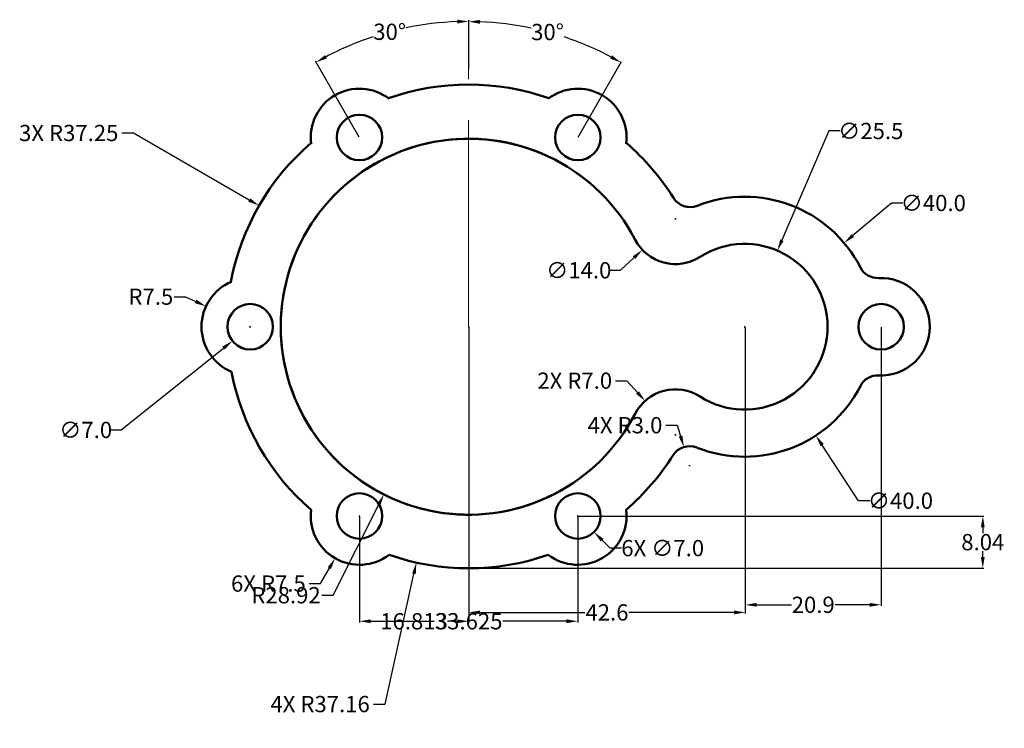
# Model space of a CAD drawing. Units: millimetres. Extents: x -471 to -319, y 2 to 111.
import ezdxf

# ---------------------------------------------------------------- set-up
doc = ezdxf.new("R2010")
doc.units = ezdxf.units.MM
doc.header["$MEASUREMENT"] = 0
doc.linetypes.add('CENTER', pattern=[50.8, 31.75, -6.35, 6.35, -6.35])
for name, color, linetype, lineweight in [('M-CNTR', 4, 'CENTER', 18), ('M-DIMS', 2, 'Continuous', 25), ('M-OUTL', 7, 'Continuous', 50)]:
    doc.layers.add(name, color=color, linetype=linetype, lineweight=lineweight)
doc.styles.get("Standard").update_dxf_attribs({"font": 'arial.ttf'})
doc.dimstyles.get("Standard").update_dxf_attribs({"dimtxt": 2.5, "dimasz": 1.75, "dimexe": 0.18, "dimexo": 0.0625, "dimgap": 0.09, "dimtad": 0, "dimtih": 1, "dimtoh": 1, "dimdec": 1, "dimzin": 0, "dimdsep": 46, "dimtxsty": 'Standard', "dimcen": 0.09, "dimadec": 0, "dimazin": 0, "dimtfac": 1, "dimtdec": 1, "dimtofl": 0, "dimtmove": 0, "dimatfit": 3, "dimfxl": 1, "dimtolj": 1, "dimtzin": 0, "dimarcsym": 0})

# ---------------------------------------------------------------- blocks, each defined once
blk = doc.blocks.new('*D1')
at = {"layer": 'Defpoints', "color": 0, "transparency": 16777216}
for p in [(-442.39, 67.1), (-435.58, 63.95)]:
    blk.add_point(p, dxfattribs=at)
at = {"layer": 'M-DIMS', "color": 0, "lineweight": -2, "transparency": 16777216}
for p, q in [((-447.31, 68.57), (-445.56, 68.57)), ((-445.56, 68.57), (-443.97, 67.83)), ((-435.67, 63.95), (-435.49, 63.95)), ((-435.58, 63.86), (-435.58, 64.04))]:
    blk.add_line(p, q, dxfattribs=at)
at = {"layer": 'M-DIMS', "color": 0, "transparency": 16777216}
blk.add_solid([(-443.85, 68.1), (-444.1, 67.57), (-442.39, 67.1)], dxfattribs=at)
at = {"layer": 'M-DIMS', "color": 0, "transparency": 16777216, "insert": (-450.88, 68.57), "char_height": 2.5, "attachment_point": 5}
blk.add_mtext('\\A1;R7.5', dxfattribs=at)
blk = doc.blocks.new('*D2')
at = {"layer": 'Defpoints', "color": 0, "transparency": 16777216}
for p in [(-432.85, 66.13), (-438.31, 61.76)]:
    blk.add_point(p, dxfattribs=at)
at = {"layer": 'M-DIMS', "color": 0, "lineweight": -2, "transparency": 16777216}
for p, q in [((-435.67, 63.95), (-435.49, 63.95)), ((-435.58, 63.86), (-435.58, 64.04)), ((-455.44, 48.07), (-439.68, 60.67)), ((-457.19, 48.07), (-455.44, 48.07))]:
    blk.add_line(p, q, dxfattribs=at)
at = {"layer": 'M-DIMS', "color": 0, "transparency": 16777216}
blk.add_solid([(-439.86, 60.9), (-439.5, 60.44), (-438.31, 61.76)], dxfattribs=at)
at = {"layer": 'M-DIMS', "color": 0, "transparency": 16777216, "insert": (-460.91, 48.07), "char_height": 2.5, "attachment_point": 5}
blk.add_mtext('\\A1;∅7.0', dxfattribs=at)
blk = doc.blocks.new('*D3')
at = {"layer": 'Defpoints', "color": 0, "transparency": 16777216}
for p in [(-365.02, 85.37), (-375.21, 75.78)]:
    blk.add_point(p, dxfattribs=at)
at = {"layer": 'M-DIMS', "color": 0, "lineweight": -2, "transparency": 16777216}
for p, q in [((-370.2, 80.57), (-370.02, 80.57)), ((-370.11, 80.48), (-370.11, 80.66)), ((-378.56, 72.63), (-376.49, 74.58)), ((-380.31, 72.63), (-378.56, 72.63))]:
    blk.add_line(p, q, dxfattribs=at)
at = {"layer": 'M-DIMS', "color": 0, "transparency": 16777216}
blk.add_solid([(-376.69, 74.79), (-376.29, 74.37), (-375.21, 75.78)], dxfattribs=at)
at = {"layer": 'M-DIMS', "color": 0, "transparency": 16777216, "insert": (-385, 72.63), "char_height": 2.5, "attachment_point": 5}
blk.add_mtext('\\A1;∅14.0', dxfattribs=at)
blk = doc.blocks.new('*D4')
at = {"layer": 'Defpoints', "color": 0, "transparency": 16777216}
for p in [(-354.42, 75.66), (-364.49, 52.24)]:
    blk.add_point(p, dxfattribs=at)
at = {"layer": 'M-DIMS', "color": 0, "lineweight": -2, "transparency": 16777216}
for p, q in [((-346.5, 94.06), (-353.72, 77.27)), ((-344.75, 94.06), (-346.5, 94.06)), ((-359.54, 63.95), (-359.36, 63.95)), ((-359.45, 63.86), (-359.45, 64.04))]:
    blk.add_line(p, q, dxfattribs=at)
at = {"layer": 'M-DIMS', "color": 0, "transparency": 16777216}
blk.add_solid([(-353.99, 77.38), (-353.46, 77.15), (-354.42, 75.66)], dxfattribs=at)
at = {"layer": 'M-DIMS', "color": 0, "transparency": 16777216, "insert": (-340.05, 94.06), "char_height": 2.5, "attachment_point": 5}
blk.add_mtext('\\A1;∅25.5', dxfattribs=at)
blk = doc.blocks.new('*D5')
at = {"layer": 'Defpoints', "color": 0, "transparency": 16777216}
for p in [(-344.16, 76.83), (-374.75, 51.06)]:
    blk.add_point(p, dxfattribs=at)
at = {"layer": 'M-DIMS', "color": 0, "lineweight": -2, "transparency": 16777216}
for p, q in [((-336.86, 82.98), (-342.82, 77.96)), ((-335.11, 82.98), (-336.86, 82.98)), ((-359.54, 63.95), (-359.36, 63.95)), ((-359.45, 63.86), (-359.45, 64.04))]:
    blk.add_line(p, q, dxfattribs=at)
at = {"layer": 'M-DIMS', "color": 0, "transparency": 16777216}
blk.add_solid([(-343.01, 78.18), (-342.63, 77.74), (-344.16, 76.83)], dxfattribs=at)
at = {"layer": 'M-DIMS', "color": 0, "transparency": 16777216, "insert": (-330.42, 82.98), "char_height": 2.5, "attachment_point": 5}
blk.add_mtext('\\A1;∅40.0', dxfattribs=at)
blk = doc.blocks.new('*D6')
at = {"layer": 'Defpoints', "color": 0, "transparency": 16777216}
for p in [(-401.95, 63.95), (-359.36, 63.95), (-359.36, 20)]:
    blk.add_point(p, dxfattribs=at)
at = {"layer": 'M-DIMS', "color": 0, "lineweight": -2, "transparency": 16777216}
for p, q in [((-401.95, 63.89), (-401.95, 19.82)), ((-359.36, 63.89), (-359.36, 19.82)), ((-400.2, 20), (-384.05, 20)), ((-361.11, 20), (-377.27, 20))]:
    blk.add_line(p, q, dxfattribs=at)
at = {"layer": 'M-DIMS', "color": 0, "transparency": 16777216}
for points in [[(-400.2, 20.29), (-400.2, 19.71), (-401.95, 20)], [(-361.11, 20.29), (-361.11, 19.71), (-359.36, 20)]]:
    blk.add_solid(points, dxfattribs=at)
at = {"layer": 'M-DIMS', "color": 0, "transparency": 16777216, "insert": (-380.66, 20), "char_height": 2.5, "attachment_point": 5}
blk.add_mtext('\\A1;42.6', dxfattribs=at)
blk = doc.blocks.new('*D7')
at = {"layer": 'Defpoints', "color": 0, "transparency": 16777216}
for p in [(-359.36, 63.95), (-338.45, 63.95), (-338.45, 21.17)]:
    blk.add_point(p, dxfattribs=at)
at = {"layer": 'M-DIMS', "color": 0, "lineweight": -2, "transparency": 16777216}
for p, q in [((-359.36, 63.89), (-359.36, 20.99)), ((-338.45, 63.89), (-338.45, 20.99)), ((-357.61, 21.17), (-352.27, 21.17)), ((-340.2, 21.17), (-345.55, 21.17))]:
    blk.add_line(p, q, dxfattribs=at)
at = {"layer": 'M-DIMS', "color": 0, "transparency": 16777216}
for points in [[(-357.61, 21.46), (-357.61, 20.88), (-359.36, 21.17)], [(-340.2, 21.46), (-340.2, 20.88), (-338.45, 21.17)]]:
    blk.add_solid(points, dxfattribs=at)
at = {"layer": 'M-DIMS', "color": 0, "transparency": 16777216, "insert": (-348.91, 21.17), "char_height": 2.5, "attachment_point": 5}
blk.add_mtext('\\A1;20.9', dxfattribs=at)
blk = doc.blocks.new('*D8')
at = {"layer": 'Defpoints', "color": 0, "transparency": 16777216}
for p in [(-410.11, 110.21), (-401.95, 103.42), (-418.77, 93.07), (-401.95, 63.95), (-401.95, 63.95)]:
    blk.add_point(p, dxfattribs=at)
at = {"layer": 'M-DIMS', "color": 0, "lineweight": -2, "transparency": 16777216}
for p, q in [((-401.95, 103.49), (-401.95, 111.1)), ((-418.8, 93.12), (-425.53, 104.78))]:
    blk.add_line(p, q, dxfattribs=at)
for start, end in [(92.1348, 101.8127), (108.2356, 117.8652)]:
    blk.add_arc((-401.95, 63.95), 46.97, start, end, dxfattribs=at)
at = {"layer": 'M-DIMS', "color": 0, "transparency": 16777216}
for points in [[(-403.71, 111.18), (-403.7, 110.59), (-401.95, 110.92)], [(-423.77, 105.22), (-424.05, 105.73), (-425.44, 104.63)]]:
    blk.add_solid(points, dxfattribs=at)
at = {"layer": 'M-DIMS', "color": 0, "transparency": 16777216, "insert": (-414.11, 109.32), "char_height": 2.5, "attachment_point": 5}
blk.add_mtext('\\A1;30°', dxfattribs=at)
blk = doc.blocks.new('*D9')
at = {"layer": 'Defpoints', "color": 0, "transparency": 16777216}
for p in [(-385.9, 108.05), (-401.95, 103.42), (-385.14, 93.07), (-401.95, 63.95), (-401.95, 63.95)]:
    blk.add_point(p, dxfattribs=at)
at = {"layer": 'M-DIMS', "color": 0, "lineweight": -2, "transparency": 16777216}
for p, q in [((-401.95, 103.49), (-401.95, 111.06)), ((-385.11, 93.12), (-378.4, 104.75))]:
    blk.add_line(p, q, dxfattribs=at)
for start, end in [(78.19, 87.8633), (62.1367, 71.7616)]:
    blk.add_arc((-401.95, 63.95), 46.93, start, end, dxfattribs=at)
at = {"layer": 'M-DIMS', "color": 0, "transparency": 16777216}
for points in [[(-400.21, 110.55), (-400.2, 111.14), (-401.95, 110.88)], [(-379.88, 105.69), (-380.16, 105.18), (-378.49, 104.59)]]:
    blk.add_solid(points, dxfattribs=at)
at = {"layer": 'M-DIMS', "color": 0, "transparency": 16777216, "insert": (-389.81, 109.28), "char_height": 2.5, "attachment_point": 5}
blk.add_mtext('\\A1;30°', dxfattribs=at)
blk = doc.blocks.new('MOUNTING-TAB-D7-R7_5')
blk.add_circle((0, 0), 3.5)
blk.add_arc((0, 0), 7.5, 112.6198, 247.3802)
blk = doc.blocks.new('*D11')
at = {"layer": 'Defpoints', "color": 0, "transparency": 16777216}
for p in [(-418.77, 34.83), (-385.14, 34.83), (-385.14, 18.64)]:
    blk.add_point(p, dxfattribs=at)
at = {"layer": 'M-DIMS', "color": 0, "lineweight": -2, "transparency": 16777216}
for p, q in [((-418.77, 34.77), (-418.77, 18.46)), ((-385.14, 34.77), (-385.14, 18.46)), ((-417.02, 18.64), (-407.24, 18.64)), ((-386.89, 18.64), (-396.67, 18.64))]:
    blk.add_line(p, q, dxfattribs=at)
at = {"layer": 'M-DIMS', "color": 0, "transparency": 16777216}
for points in [[(-417.02, 18.93), (-417.02, 18.35), (-418.77, 18.64)], [(-386.89, 18.93), (-386.89, 18.35), (-385.14, 18.64)]]:
    blk.add_solid(points, dxfattribs=at)
at = {"layer": 'M-DIMS', "color": 0, "transparency": 16777216, "insert": (-401.95, 18.64), "char_height": 2.5, "attachment_point": 5}
blk.add_mtext('\\A1;33.625', dxfattribs=at)
blk = doc.blocks.new('*D12')
at = {"layer": 'Defpoints', "color": 0, "transparency": 16777216}
for p in [(-418.77, 34.83), (-401.95, 26.79), (-401.95, 18.64)]:
    blk.add_point(p, dxfattribs=at)
at = {"layer": 'M-DIMS', "color": 0, "lineweight": -2, "transparency": 16777216}
for p, q in [((-418.77, 34.77), (-418.77, 18.46)), ((-401.95, 26.73), (-401.95, 18.46)), ((-417.02, 18.64), (-415.52, 18.64)), ((-403.7, 18.64), (-405.2, 18.64))]:
    blk.add_line(p, q, dxfattribs=at)
at = {"layer": 'M-DIMS', "color": 0, "transparency": 16777216}
for points in [[(-417.02, 18.93), (-417.02, 18.35), (-418.77, 18.64)], [(-403.7, 18.93), (-403.7, 18.35), (-401.95, 18.64)]]:
    blk.add_solid(points, dxfattribs=at)
at = {"layer": 'M-DIMS', "color": 0, "transparency": 16777216, "insert": (-410.36, 18.64), "char_height": 2.5, "attachment_point": 5}
blk.add_mtext('\\A1;16.813', dxfattribs=at)
blk = doc.blocks.new('*D13')
at = {"layer": 'Defpoints', "color": 0, "transparency": 16777216}
for p in [(-385.14, 34.83), (-401.95, 26.79), (-322.8, 26.79)]:
    blk.add_point(p, dxfattribs=at)
at = {"layer": 'M-DIMS', "color": 0, "lineweight": -2, "transparency": 16777216}
for p, q in [((-385.08, 34.83), (-322.62, 34.83)), ((-322.8, 33.08), (-322.8, 32.17)), ((-322.8, 28.54), (-322.8, 29.44)), ((-401.89, 26.79), (-322.62, 26.79))]:
    blk.add_line(p, q, dxfattribs=at)
at = {"layer": 'M-DIMS', "color": 0, "transparency": 16777216}
for points in [[(-323.1, 33.08), (-322.51, 33.08), (-322.8, 34.83)], [(-323.1, 28.54), (-322.51, 28.54), (-322.8, 26.79)]]:
    blk.add_solid(points, dxfattribs=at)
at = {"layer": 'M-DIMS', "color": 0, "transparency": 16777216, "insert": (-322.8, 30.81), "char_height": 2.5, "attachment_point": 5}
blk.add_mtext('\\A1;8.04', dxfattribs=at)
blk = doc.blocks.new('*D14')
at = {"layer": 'Defpoints', "color": 0, "transparency": 16777216}
for p in [(-387.62, 37.3), (-382.66, 32.36)]:
    blk.add_point(p, dxfattribs=at)
at = {"layer": 'M-DIMS', "color": 0, "lineweight": -2, "transparency": 16777216}
for p, q in [((-385.14, 34.74), (-385.14, 34.92)), ((-385.23, 34.83), (-385.05, 34.83)), ((-380.18, 29.89), (-381.42, 31.13)), ((-378.43, 29.89), (-380.18, 29.89))]:
    blk.add_line(p, q, dxfattribs=at)
at = {"layer": 'M-DIMS', "color": 0, "transparency": 16777216}
blk.add_solid([(-381.21, 31.33), (-381.63, 30.92), (-382.66, 32.36)], dxfattribs=at)
at = {"layer": 'M-DIMS', "color": 0, "transparency": 16777216, "insert": (-372.08, 29.89), "char_height": 2.5, "attachment_point": 5}
blk.add_mtext('\\A1;6X ∅7.0', dxfattribs=at)
blk = doc.blocks.new('*D15')
at = {"layer": 'Defpoints', "color": 0, "transparency": 16777216}
for p in [(-418.77, 34.83), (-422.52, 28.33)]:
    blk.add_point(p, dxfattribs=at)
at = {"layer": 'M-DIMS', "color": 0, "lineweight": -2, "transparency": 16777216}
for p, q in [((-418.77, 34.74), (-418.77, 34.92)), ((-418.86, 34.83), (-418.68, 34.83)), ((-424.77, 24.44), (-423.39, 26.82)), ((-426.52, 24.44), (-424.77, 24.44))]:
    blk.add_line(p, q, dxfattribs=at)
at = {"layer": 'M-DIMS', "color": 0, "transparency": 16777216}
blk.add_solid([(-423.65, 26.96), (-423.14, 26.67), (-422.52, 28.33)], dxfattribs=at)
at = {"layer": 'M-DIMS', "color": 0, "transparency": 16777216, "insert": (-432.78, 24.44), "char_height": 2.5, "attachment_point": 5}
blk.add_mtext('\\A1;6X R7.5', dxfattribs=at)
blk = doc.blocks.new('*D16')
at = {"layer": 'Defpoints', "color": 0, "transparency": 16777216}
for p in [(-434.21, 82.57), (-401.95, 63.95)]:
    blk.add_point(p, dxfattribs=at)
at = {"layer": 'M-DIMS', "color": 0, "lineweight": -2, "transparency": 16777216}
for p, q in [((-455.32, 93.75), (-453.57, 93.75)), ((-453.57, 93.75), (-435.73, 83.45)), ((-402.04, 63.95), (-401.86, 63.95)), ((-401.95, 63.86), (-401.95, 64.04))]:
    blk.add_line(p, q, dxfattribs=at)
at = {"layer": 'M-DIMS', "color": 0, "transparency": 16777216}
blk.add_solid([(-435.58, 83.7), (-435.88, 83.2), (-434.21, 82.57)], dxfattribs=at)
at = {"layer": 'M-DIMS', "color": 0, "transparency": 16777216, "insert": (-463.52, 93.75), "char_height": 2.5, "attachment_point": 5}
blk.add_mtext('\\A1;3X R37.25', dxfattribs=at)
blk = doc.blocks.new('*D17')
at = {"layer": 'Defpoints', "color": 0, "transparency": 16777216}
for p in [(-401.95, 63.95), (-410, 27.67)]:
    blk.add_point(p, dxfattribs=at)
at = {"layer": 'M-DIMS', "color": 0, "lineweight": -2, "transparency": 16777216}
for p, q in [((-402.04, 63.95), (-401.86, 63.95)), ((-401.95, 63.86), (-401.95, 64.04)), ((-414.83, 5.9), (-410.38, 25.96)), ((-416.58, 5.9), (-414.83, 5.9))]:
    blk.add_line(p, q, dxfattribs=at)
at = {"layer": 'M-DIMS', "color": 0, "transparency": 16777216}
blk.add_solid([(-410.66, 26.02), (-410.09, 25.9), (-410, 27.67)], dxfattribs=at)
at = {"layer": 'M-DIMS', "color": 0, "transparency": 16777216, "insert": (-424.82, 5.9), "char_height": 2.5, "attachment_point": 5}
blk.add_mtext('\\A1;4X R37.16', dxfattribs=at)
blk = doc.blocks.new('*D18')
at = {"layer": 'Defpoints', "color": 0, "transparency": 16777216}
for p in [(-401.95, 63.95), (-415, 38.14)]:
    blk.add_point(p, dxfattribs=at)
at = {"layer": 'M-DIMS', "color": 0, "lineweight": -2, "transparency": 16777216}
for p, q in [((-402.04, 63.95), (-401.86, 63.95)), ((-401.95, 63.86), (-401.95, 64.04)), ((-422.83, 22.65), (-415.79, 36.58)), ((-424.58, 22.65), (-422.83, 22.65))]:
    blk.add_line(p, q, dxfattribs=at)
at = {"layer": 'M-DIMS', "color": 0, "transparency": 16777216}
blk.add_solid([(-416.05, 36.71), (-415.53, 36.45), (-415, 38.14)], dxfattribs=at)
at = {"layer": 'M-DIMS', "color": 0, "transparency": 16777216, "insert": (-430.07, 22.65), "char_height": 2.5, "attachment_point": 5}
blk.add_mtext('\\A1;R28.92', dxfattribs=at)
blk = doc.blocks.new('*D19')
at = {"layer": 'Defpoints', "color": 0, "transparency": 16777216}
for p in [(-368.82, 45.45), (-367.95, 42.58)]:
    blk.add_point(p, dxfattribs=at)
at = {"layer": 'M-DIMS', "color": 0, "lineweight": -2, "transparency": 16777216}
for p, q in [((-371.59, 48.8), (-369.84, 48.8)), ((-369.84, 48.8), (-369.33, 47.12)), ((-368.04, 42.58), (-367.86, 42.58)), ((-367.95, 42.49), (-367.95, 42.67))]:
    blk.add_line(p, q, dxfattribs=at)
at = {"layer": 'M-DIMS', "color": 0, "transparency": 16777216}
blk.add_solid([(-369.05, 47.21), (-369.61, 47.04), (-368.82, 45.45)], dxfattribs=at)
at = {"layer": 'M-DIMS', "color": 0, "transparency": 16777216, "insert": (-377.88, 48.8), "char_height": 2.5, "attachment_point": 5}
blk.add_mtext('\\A1;4X R3.0', dxfattribs=at)
blk = doc.blocks.new('*D20')
at = {"layer": 'Defpoints', "color": 0, "transparency": 16777216}
for p in [(-370.41, 80.68), (-348.5, 47.22)]:
    blk.add_point(p, dxfattribs=at)
at = {"layer": 'M-DIMS', "color": 0, "lineweight": -2, "transparency": 16777216}
for p, q in [((-359.54, 63.95), (-359.36, 63.95)), ((-359.45, 63.86), (-359.45, 64.04)), ((-341.93, 37.18), (-347.54, 45.75)), ((-340.18, 37.18), (-341.93, 37.18))]:
    blk.add_line(p, q, dxfattribs=at)
at = {"layer": 'M-DIMS', "color": 0, "transparency": 16777216}
blk.add_solid([(-347.3, 45.91), (-347.79, 45.59), (-348.5, 47.22)], dxfattribs=at)
at = {"layer": 'M-DIMS', "color": 0, "transparency": 16777216, "insert": (-335.48, 37.18), "char_height": 2.5, "attachment_point": 5}
blk.add_mtext('\\A1;∅40.0', dxfattribs=at)
blk = doc.blocks.new('*D21')
at = {"layer": 'Defpoints', "color": 0, "transparency": 16777216}
for p in [(-374.79, 52.53), (-370.11, 47.32)]:
    blk.add_point(p, dxfattribs=at)
at = {"layer": 'M-DIMS', "color": 0, "lineweight": -2, "transparency": 16777216}
for p, q in [((-379.35, 55.65), (-377.6, 55.65)), ((-377.6, 55.65), (-375.96, 53.83)), ((-370.2, 47.32), (-370.02, 47.32)), ((-370.11, 47.23), (-370.11, 47.41))]:
    blk.add_line(p, q, dxfattribs=at)
at = {"layer": 'M-DIMS', "color": 0, "transparency": 16777216}
blk.add_solid([(-375.75, 54.02), (-376.18, 53.63), (-374.79, 52.53)], dxfattribs=at)
at = {"layer": 'M-DIMS', "color": 0, "transparency": 16777216, "insert": (-385.62, 55.65), "char_height": 2.5, "attachment_point": 5}
blk.add_mtext('\\A1;2X R7.0', dxfattribs=at)

msp = doc.modelspace()

# ---------------------------------------------------------------- linework, layer by layer
at = {"layer": 'M-CNTR'}
msp.add_line((-401.9544, 63.9485), (-401.9544, 103.4234), dxfattribs=at)
at = {"layer": 'M-OUTL'}
msp.add_circle((-338.4544, 63.9485), 3.5, dxfattribs=at)
msp.add_circle((-338.4544, 63.9485), 3.5, dxfattribs=at)
for centre, radius, start, end in [((-401.9544, 63.9485), 37.25, 70.644837, 109.355163), ((-401.9544, 63.9485), 28.9192, 27.572452, 310.746053), ((-401.9544, 63.9485), 28.9192, 49.253947, 332.427548), ((-401.9544, 63.9485), 37.25, 130.644837, 169.355163), ((-401.9544, 63.9485), 37.25, 32.128459, 49.355163), ((-367.8684, 85.3542), 3, 212.128459, 291.458352), ((-359.4544, 63.9485), 20, 27.125452, 111.458352), ((-370.1146, 80.5744), 7, 207.572452, 302.667248), ((-359.4544, 63.9485), 12.75, 0, 122.667248), ((-338.9842, 74.4351), 3, 207.125452, 272.892001), ((-338.4544, 63.9485), 7.5, 0, 92.892001), ((-359.4544, 63.9485), 12.75, 237.332752, 0), ((-338.4544, 63.9485), 7.5, 267.107999, 0), ((-401.9544, 63.9485), 37.1602, 190.737144, 229.262856), ((-338.9842, 53.4619), 3, 87.107999, 152.874548), ((-359.4544, 63.9485), 20, 248.541648, 332.874548), ((-370.1146, 47.3226), 7, 57.332752, 152.427548), ((-367.9533, 42.5763), 3, 68.314092, 147.847666), ((-401.9544, 63.9485), 37.1602, 310.737144, 327.847666), ((-401.9544, 63.9485), 37.1602, 310.737144, 327.847666), ((-401.9544, 63.9485), 37.1602, 250.737144, 289.262856)]:
    msp.add_arc(centre, radius, start, end, dxfattribs=at)

# ---------------------------------------------------------------- block references
for p, rotation in [((-418.7669, 93.0686), 299.9999999999989), ((-385.1419, 93.0686), 239.9999999999979), ((-418.7669, 34.8284), 59.99999999999881), ((-385.1419, 34.8284), 119.9999999999991)]:
    msp.add_blockref('MOUNTING-TAB-D7-R7_5', p, dxfattribs=dict(at, rotation=rotation))
msp.add_blockref('MOUNTING-TAB-D7-R7_5', (-435.5794, 63.9485), dxfattribs=at)

# ---------------------------------------------------------------- dimensions: what is measured, and where the dimension line sits
at = {"layer": 'M-DIMS'}
for base, line1, line2, picture, middle in [((-410.1107, 110.2051), ((-401.9544, 63.9485), (-401.9544, 103.4234)), ((-401.9544, 63.9485), (-418.7669, 93.0686)), '*D8', (-414.1112, 109.3183)), ((-385.9033, 108.0484), ((-385.1419, 93.0686), (-401.9544, 63.9485)), ((-401.9544, 63.9485), (-401.9544, 103.4234)), '*D9', (-389.808, 109.2795))]:
    dim = msp.add_angular_dim_2l(base=base, line1=line1, line2=line2, dimstyle='Standard', override={"dimclrd": 0, "dimclre": 0, "dimclrt": 0}, dxfattribs=at)
    dim.commit()
    dim.dimension.update_dxf_attribs({"geometry": picture, "text_midpoint": middle})
for center, mpoint, text, override, picture, middle in [((-401.9544, 63.9485), (-434.2141, 82.5731), '3X <>', {"dimdec": 2, "dimlfac": 1, "dimrnd": 0, "dimzin": 0, "dimdsep": 46, "dimlunit": 2}, '*D16', (-463.5187, 93.7478)), ((-401.9544, 63.9485), (-410.0001, 27.6697), '4X <>', {"dimdec": 2, "dimlfac": 1, "dimrnd": 0, "dimzin": 0, "dimdsep": 46, "dimlunit": 2}, '*D17', (-424.8172, 5.9025)), ((-370.1146, 47.3226), (-374.7945, 52.5282), '2X <>', {"dimdec": 1, "dimlfac": 1, "dimrnd": 0, "dimzin": 0, "dimdsep": 46, "dimlunit": 2}, '*D21', (-385.6173, 55.6517)), ((-418.7669, 34.8284), (-422.5178, 28.3337), '6X <>', {"dimdec": 1, "dimlfac": 1, "dimrnd": 0, "dimzin": 0, "dimdsep": 46, "dimlunit": 2}, '*D15', (-432.7825, 24.4369))]:
    dim = msp.add_radius_dim(center=center, mpoint=mpoint, text=text, dimstyle='Standard', override=override, dxfattribs=at)
    dim.commit()
    dim.dimension.update_dxf_attribs({"geometry": picture, "text_midpoint": middle, "dimtype": 164})
for p1, p2, override, picture, middle in [((-364.4925, 52.2361), (-354.4163, 75.6609), {"dimclrd": 0, "dimclre": 0, "dimclrt": 0}, '*D4', (-340.0474, 94.0555)), ((-365.0172, 85.3719), (-375.2121, 75.7769), {"dimclrd": 0, "dimclre": 0, "dimclrt": 0}, '*D3', (-385.0007, 72.6279)), ((-374.75, 51.0626), (-344.1588, 76.8344), {"dimclrd": 0, "dimclre": 0, "dimclrt": 0}, '*D5', (-330.4206, 82.9806)), ((-370.4091, 80.6815), (-348.4997, 47.2154), {"dimdec": 1, "dimlfac": 1, "dimrnd": 0, "dimzin": 0, "dimdsep": 46, "dimlunit": 2}, '*D20', (-335.4843, 37.1756)), ((-432.8456, 66.134), (-438.3132, 61.7629), {"dimclrd": 0, "dimclre": 0, "dimclrt": 0}, '*D2', (-460.9118, 48.0704))]:
    dim = msp.add_diameter_dim_2p(p1=p1, p2=p2, dimstyle='Standard', override=override, dxfattribs=at)
    dim.commit()
    dim.dimension.update_dxf_attribs({"geometry": picture, "text_midpoint": middle, "dimtype": 163})
dim = msp.add_radius_dim(center=(-435.5794, 63.9485), mpoint=(-442.3862, 67.0977), dimstyle='Standard', override={"dimclrd": 0, "dimclre": 0, "dimclrt": 0}, dxfattribs=at)
dim.commit()
dim.dimension.update_dxf_attribs({"geometry": '*D1', "text_midpoint": (-450.8841, 68.5673)})
dim = msp.add_radius_dim(center=(-401.9544, 63.9485), mpoint=(-415.0004, 38.1391), dimstyle='Standard', override={"dimdec": 2, "dimlfac": 1, "dimrnd": 0, "dimzin": 0, "dimdsep": 46, "dimlunit": 2}, dxfattribs=at)
dim.commit()
dim.dimension.update_dxf_attribs({"geometry": '*D18', "text_midpoint": (-430.0697, 22.6535), "dimtype": 164})
for base, p1, p2, override, picture, middle in [((-359.3644, 20.0031), (-401.9544, 63.9485), (-359.3644, 63.9485), {"dimclrd": 0, "dimclre": 0, "dimclrt": 0}, '*D6', (-380.6594, 20.0031)), ((-338.4544, 21.1714), (-359.3644, 63.9485), (-338.4544, 63.9485), {"dimclrd": 0, "dimclre": 0, "dimclrt": 0}, '*D7', (-348.9094, 21.1714)), ((-385.1419, 18.6383), (-418.7669, 34.8284), (-385.1419, 34.8284), {"dimdec": 3, "dimlfac": 1, "dimrnd": 0, "dimzin": 0, "dimdsep": 46, "dimlunit": 2}, '*D11', (-401.9544, 18.6383)), ((-401.954403, 18.638284), (-418.766903, 34.828382), (-401.954403, 26.788284), {"dimdec": 3, "dimlfac": 1, "dimrnd": 0, "dimzin": 0, "dimdsep": 46, "dimlunit": 2}, '*D12', (-410.360653, 18.638284))]:
    dim = msp.add_linear_dim(base=base, p1=p1, p2=p2, dimstyle='Standard', override=override, dxfattribs=at)
    dim.commit()
    dim.dimension.update_dxf_attribs({"geometry": picture, "text_midpoint": middle})
dim = msp.add_radius_dim(center=(-367.9533, 42.5763), mpoint=(-368.8228, 45.4476), text='4X <>', dimstyle='Standard', override={"dimdec": 1, "dimlfac": 1, "dimrnd": 0, "dimzin": 0, "dimdsep": 46, "dimlunit": 2}, dxfattribs=at)
dim.commit()
dim.dimension.update_dxf_attribs({"geometry": '*D19', "text_midpoint": (-377.8812, 48.7973)})
dim = msp.add_diameter_dim_2p(p1=(-387.6235, 37.2965), p2=(-382.6603, 32.3603), text='6X <>', dimstyle='Standard', override={"dimdec": 1, "dimlfac": 1, "dimrnd": 0, "dimzin": 0, "dimdsep": 46, "dimlunit": 2}, dxfattribs=at)
dim.commit()
dim.dimension.update_dxf_attribs({"geometry": '*D14', "text_midpoint": (-372.081, 29.8922), "dimtype": 163})
dim = msp.add_linear_dim(base=(-322.8044, 26.7883), p1=(-385.1419, 34.8284), p2=(-401.9544, 26.7883), angle=90, dimstyle='Standard', override={"dimdec": 2, "dimlfac": 1, "dimrnd": 0, "dimzin": 0, "dimdsep": 46, "dimlunit": 2}, dxfattribs=at)
dim.commit()
dim.dimension.update_dxf_attribs({"geometry": '*D13', "text_midpoint": (-322.8044, 30.8083)})

doc.saveas('drawing.dxf')
